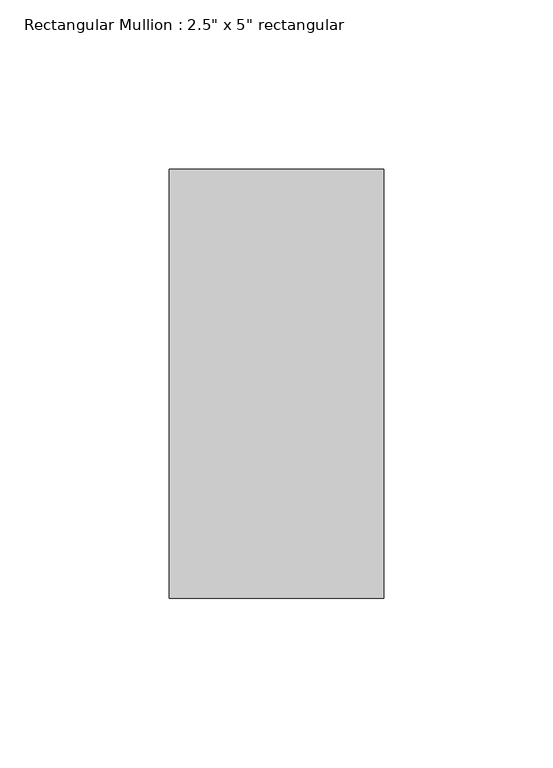
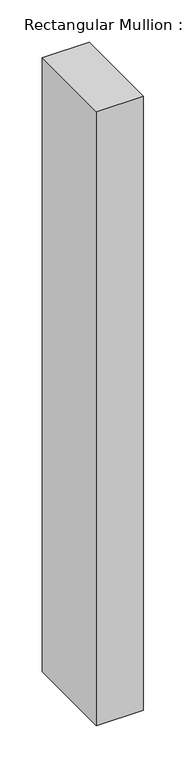
"""IFC4 building model written with IfcOpenShell, lengths in millimetres: member geometry."""

from ifc_helpers import new_model, si_unit, frame, origin, place, context, project, spatial, polyline, outline, extrude, source, transform, mapped, element, save


def member_5cd4c5ac(model_context):
    return source(origin(), model_context, "Body", "SweptSolid", [
        extrude(outline(polyline([(0.0, 63.5), (0.0, -63.5), (-63.5, -63.5), (-63.5, 63.5), (0.0, 63.5)])), frame((0.0, 0.0, -882.65), z_axis=(0.0, 0.0, 1.0), x_axis=(1.0, 0.0, 0.0)), (0.0, 0.0, 1.0), 882.65),
    ])


if __name__ == "__main__":
    model = new_model("IFC4")
    model_context = context("Model", 3, world=origin())
    ifc_project = project(units=[si_unit("LENGTHUNIT", "METRE", prefix="MILLI")], contexts=[model_context])
    site = spatial("IfcSite", under=ifc_project)
    building = spatial("IfcBuilding", under=site)
    placement = place(None, origin())
    member_shape = member_5cd4c5ac(model_context)
    element("IfcMember", 1, ObjectType="Rectangular Mullion : 2.5\" x 5\" rectangular", at=placement, inside=building, context=model_context, shape_type="MappedRepresentation", body=[
        mapped(member_shape, transform((0.0, 0.0, 0.0), x_axis=(1.0, 0.0, 0.0), y_axis=(0.0, 1.0, 0.0), z_axis=(0.0, 0.0, 1.0))),
    ])
    save(model, "model.ifc")

# Revit data of these elements
# Type "Rectangular Mullion : 2.5\" x 5\" rectangular"
#   built-in parameter 1007304 = 0.416667 (stored number, unit not read)
#   built-in parameter 1007301 = 0.104167 (stored number, unit not read)
#   built-in parameter 1007300 = 0.104167 (stored number, unit not read)
# Element 1 (IfcMember, "Rectangular Mullion : 2.5\" x 5\" rectangular")
#   Materials on its faces: "Aluminum"
# Materials
#   "Aluminum": class "Metal", colour RGB 247 247 247, transparency 0, Description = "Aluminum 6061", Cost = 0
